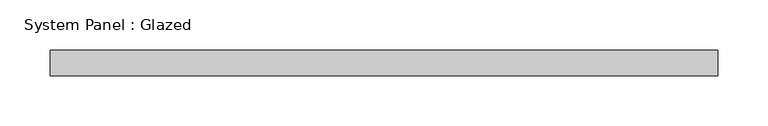
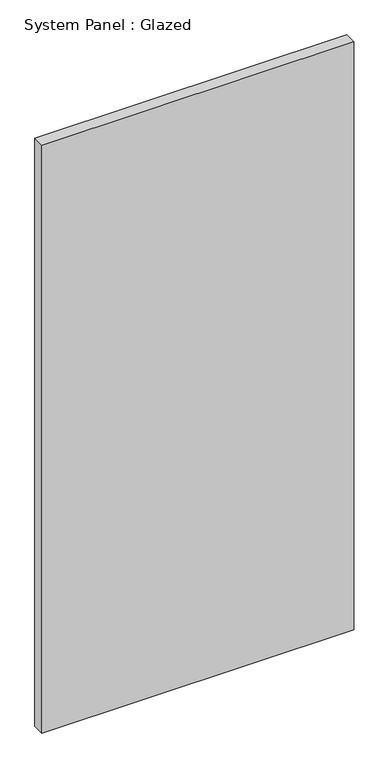
"""IFC4 building model written with IfcOpenShell, lengths in millimetres: plate geometry, System Panel : Glazed."""

from ifc_helpers import new_model, si_unit, origin, origin_with_axes, place, context, project, spatial, polyline, outline, extrude, source, transform, mapped, element, save


def system_panel_glazed_125786c9(model_context):
    return source(origin(), model_context, "Body", "SweptSolid", [
        extrude(outline(polyline([(333.375, 19.05), (-333.375, 19.05), (-333.375, 44.45), (333.375, 44.45), (333.375, 19.05)])), origin_with_axes(), (0.0, 0.0, 1.0), 1328.9654832),
    ])


if __name__ == "__main__":
    model = new_model("IFC4")
    model_context = context("Model", 3, world=origin())
    ifc_project = project(units=[si_unit("LENGTHUNIT", "METRE", prefix="MILLI")], contexts=[model_context])
    site = spatial("IfcSite", under=ifc_project)
    building = spatial("IfcBuilding", under=site)
    placement = place(None, origin())
    system_panel_glazed_shape = system_panel_glazed_125786c9(model_context)
    element("IfcPlate", 1, ObjectType="System Panel : Glazed", at=placement, inside=building, context=model_context, shape_type="MappedRepresentation", body=[
        mapped(system_panel_glazed_shape, transform((0.0, 0.0, 0.0), x_axis=(1.0, 0.0, 0.0), y_axis=(0.0, 1.0, 0.0), z_axis=(0.0, 0.0, 1.0))),
    ])
    save(model, "model.ifc")

# Revit data of these elements
# Type "System Panel : Glazed"
#   Construction Type Id = "GSP4R"
#   Analytic Construction = "1/8 in Pilkington single glazing"
#   Visual Light Transmittance = 0.9
#   Solar Heat Gain Coefficient = 0.86
#   Heat Transfer Coefficient (U) = 1.18115 BTU/(h·ft²·°F)
#   Define Thermal Properties by = 1
# Element 1 (IfcPlate, "System Panel : Glazed")
#   Materials on its faces: "Glass"
# Materials
#   "Glass": class "Glass", colour RGB 0 128 192, transparency 0.75, Description = "Soda Lime Glass", Cost = 0
